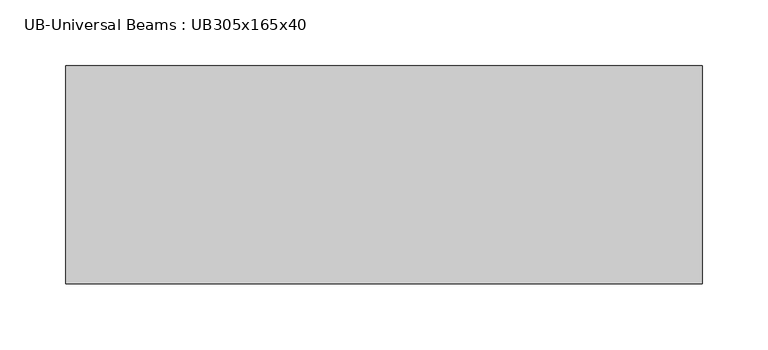
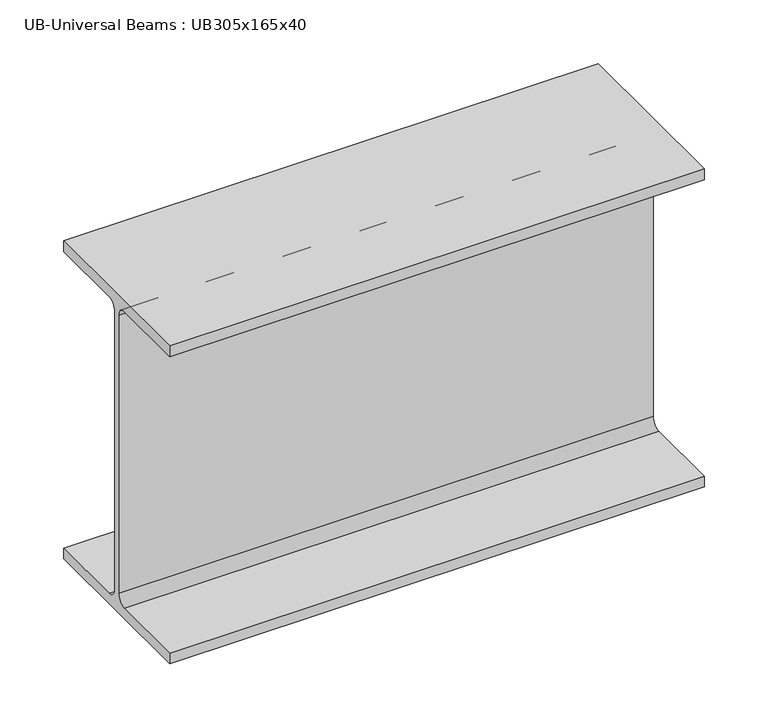
"""IFC4 building model written with IfcOpenShell, lengths in millimetres: beam geometry, UB-Universal Beams : UB305x165x40."""

from ifc_helpers import new_model, si_unit, point, frame, frame_2d, origin, place, context, project, spatial, polyline, circle_curve, trimmed, segment, composite_curve, outline, extrude, source, transform, mapped, element, save


def ub_universal_beams_ub305x165x40_3f5046e3(model_context):
    return source(origin(), model_context, "Body", "SweptSolid", [
        extrude(outline(composite_curve([segment(polyline([(82.5, -141.5), (82.5, -151.7), (-82.5, -151.7), (-82.5, -141.5), (-11.9, -141.5)]), True, "CONTINUOUS"), segment(trimmed(circle_curve(frame_2d((-11.9, -132.6)), 8.9), [point((-11.9, -141.5))], [point((-3.0, -132.6))], True, "CARTESIAN"), True, "CONTINUOUS"), segment(polyline([(-3.0, -132.6), (-3.0, 132.6)]), True, "CONTINUOUS"), segment(trimmed(circle_curve(frame_2d((-11.9, 132.6)), 8.9), [point((-3.0, 132.6))], [point((-11.9, 141.5))], True, "CARTESIAN"), True, "CONTINUOUS"), segment(polyline([(-11.9, 141.5), (-82.5, 141.5), (-82.5, 151.7), (82.5, 151.7), (82.5, 141.5), (11.9, 141.5)]), True, "CONTINUOUS"), segment(trimmed(circle_curve(frame_2d((11.9, 132.6)), 8.9), [point((11.9, 141.5))], [point((3.0, 132.6))], True, "CARTESIAN"), True, "CONTINUOUS"), segment(polyline([(3.0, 132.6), (3.0, -132.6)]), True, "CONTINUOUS"), segment(trimmed(circle_curve(frame_2d((11.9, -132.6)), 8.9), [point((3.0, -132.6))], [point((11.9, -141.5))], True, "CARTESIAN"), True, "CONTINUOUS"), segment(polyline([(11.9, -141.5), (82.5, -141.5)]), True, "CONTINUOUS")], self_intersect=False)), frame((-252.25, 0.0, 0.0), z_axis=(1.0, 0.0, 0.0), x_axis=(0.0, 1.0, 0.0)), (0.0, 0.0, 1.0), 482.3),
    ])


if __name__ == "__main__":
    model = new_model("IFC4")
    model_context = context("Model", 3, world=origin())
    ifc_project = project(units=[si_unit("LENGTHUNIT", "METRE", prefix="MILLI")], contexts=[model_context])
    site = spatial("IfcSite", under=ifc_project)
    building = spatial("IfcBuilding", under=site)
    placement = place(None, origin())
    ub_universal_beams_ub305x165x40_shape = ub_universal_beams_ub305x165x40_3f5046e3(model_context)
    element("IfcBeam", 1, ObjectType="UB-Universal Beams : UB305x165x40", at=placement, inside=building, context=model_context, shape_type="MappedRepresentation", body=[
        mapped(ub_universal_beams_ub305x165x40_shape, transform((0.0, 0.0, 0.0), x_axis=(1.0, 0.0, 0.0), y_axis=(0.0, 1.0, 0.0), z_axis=(0.0, 0.0, 1.0))),
    ])
    save(model, "model.ifc")

# Revit data of these elements
# Type "UB-Universal Beams : UB305x165x40"
#   Section Name Key = "UB305X165X40"
#   Width = 16.5 cm
#   Web Thickness = 0.6 cm
#   Web Fillet = 0.89 cm
#   Warping Constant = 164000.0 cm⁶
#   Torsional Moment of Inertia = 14.70 cm⁴
#   Section Area = 51.3 cm²
#   Plastic Modulus weak axis = 142.0 cm³
#   Plastic Modulus strong axis = 623.0 cm³
#   Nominal Weight = 40.2999 kgf/m
#   Moment of Inertia weak axis = 764.00 cm⁴
#   Moment of Inertia strong axis = 8503.00 cm⁴
#   Height = 30.34 cm
#   Flange Thickness = 1.02 cm
#   Elastic Modulus weak axis = 92.6 cm³
#   Elastic Modulus strong axis = 560.0 cm³
#   Centroid Vertical = 15.17 cm
#   Centroid Horizontal = 8.25 cm
#   Bolt Spacing = 9.0 cm
#   Length [instance default] = 1500 mm
#   Structural Material [instance default] = Metal - Steel 43-275
#   Type Comments = ""
#   Assembly Code = ""
# Element 1 (IfcBeam, "UB-Universal Beams : UB305x165x40")
#   Materials on its faces: "Metal - Steel 43-275"
# Materials
#   "Metal - Steel 43-275": class "Metal", colour RGB 247 247 247, transparency 0, Cost = 0
